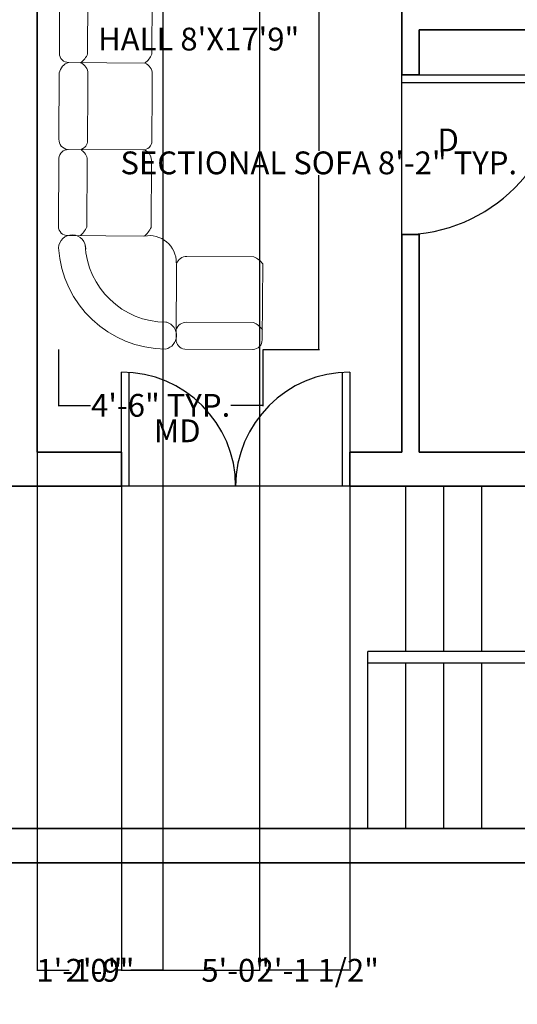
# Model space of a CAD drawing. Units: inches. Extents: x -26 to 575, y -18 to 513.
# Tile 15 of 28: x 274 to 405, y -18 to 241. Entities that reach past the tile are written whole.
import ezdxf

# ---------------------------------------------------------------- set-up
doc = ezdxf.new("R2010")
doc.units = ezdxf.units.IN
doc.header["$MEASUREMENT"] = 0
for name, color, linetype, lineweight in [('A-ANNO-DIMS', 2, 'Continuous', 18), ('A-ANNO-TEXT', 7, 'Continuous', 18), ('A-AREA-IDEN', 7, 'Continuous', 18), ('A-DOOR', 3, 'Continuous', 25), ('A-FLOR-STRS', 7, 'Continuous', 25), ('A-WALL', 7, 'Continuous', 35), ('Furniture', 8, 'Continuous', 15)]:
    doc.layers.add(name, color=color, linetype=linetype, lineweight=lineweight)
doc.styles.get("Standard").update_dxf_attribs({"font": 'arial.ttf', "height": 6})
doc.dimstyles.get("Standard").update_dxf_attribs({"dimtxt": 6, "dimasz": 0.18, "dimexe": 0.18, "dimexo": 0.0625, "dimgap": 0.09, "dimtad": 0, "dimtih": 1, "dimtoh": 1, "dimzin": 0, "dimdsep": 46, "dimlunit": 3, "dimtxsty": 'Standard', "dimcen": 0.09, "dimadec": 0, "dimazin": 0, "dimtfac": 1, "dimtofl": 0, "dimtmove": 0, "dimatfit": 3, "dimfxl": 1, "dimtolj": 1, "dimtzin": 0, "dimarcsym": 0})

# ---------------------------------------------------------------- blocks, each defined once
blk = doc.blocks.new('SOFA-L-SECTIONAL')
for p, q in [((0.33, 95.83, -13.5), (0.23, 77.86, -13.5)), ((22.74, 97.99, -13.5), (2.82, 98.09, -13.5)), ((7.68, 77.72, -13.5), (7.77, 95.38, -13.5)), ((24.59, 77.63, -13.5), (24.69, 95.29, -13.5)), ((2.7, 75.47, -13.5), (22.72, 75.27, -13.5)), ((0.21, 72.7, -13.5), (0.12, 55.25, -13.5)), ((7.74, 68.12, -13.5), (7.76, 72.56, -13.5)), ((24.65, 68.03, -13.5), (24.67, 72.47, -13.5)), ((7.67, 54.9, -13.5), (7.74, 68.12, -13.5)), ((24.58, 54.81, -13.5), (24.65, 68.03, -13.5)), ((2.38, 52.55, -13.5), (22.19, 52.45, -13.5)), ((22.5, 52.45, -13.5), (2.58, 52.55, -13.5)), ((0.09, 50.29, -13.5), (0, 32.32, -13.5)), ((7.45, 32.18, -13.5), (7.54, 49.84, -13.5)), ((24.36, 32.09, -13.5), (24.45, 49.75, -13.5)), ((2.47, 29.93, -13.5), (22.49, 29.73, -13.5)), ((51.42, 24.36, -13.5), (33.76, 24.45, -13.5)), ((31.06, 22.5, -13.5), (30.96, 2.58, -13.5)), ((53.78, 22.49, -13.5), (53.58, 2.47, -13.5)), ((28.5, 7.13, -13.5), (28.26, 7.13, -13.5)), ((30.97, 5.19, -13.5), (30.97, 5.12, -13.5)), ((51.33, 7.05, -13.5), (33.67, 7.14, -13.5)), ((33.22, 0.09, -13.5), (51.19, 0, -13.5))]:
    blk.add_line(p, q)
for centre, radius, start, end in [((2.8, 95.6, -13.5), 2.49, 89.7045, 174.7543), ((4.96, 95.39, -13.5), 2.82, 359.7045, 63.7788), ((21.87, 95.31, -13.5), 2.82, 359.7045, 71.9933), ((2.61, 77.85, -13.5), 2.38, 179.7045, 272.1133), ((2.36, 80.01, -13.5), 5.79, 306.5883, 336.7547), ((3.67, 72.1, -13.5), 3.51, 105.9725, 170.1982), ((4.8, 72.57, -13.5), 2.96, 359.7045, 69.9456), ((19.27, 79.92, -13.5), 5.79, 306.5883, 336.7547), ((21.71, 72.48, -13.5), 2.96, 359.7045, 69.9456), ((2.84, 55.23, -13.5), 2.72, 179.7045, 260.1487), ((5.3, 54.91, -13.5), 2.37, 286.4623, 359.7335), ((22.21, 54.82, -13.5), 2.37, 269.7045, 359.7335), ((2.57, 50.06, -13.5), 2.49, 89.7045, 174.7543), ((4.72, 49.86, -13.5), 2.82, 359.7045, 63.7788), ((21.63, 49.77, -13.5), 2.82, 359.7045, 71.9933), ((2.38, 32.31, -13.5), 2.38, 179.7045, 272.1133), ((2.12, 34.47, -13.5), 5.79, 306.5883, 336.7547), ((19.04, 34.38, -13.5), 5.79, 306.5883, 336.7547), ((3.6, 26.52, -13.5), 3.6, 357.7166, 177.7166), ((23.89, 22.8, -13.5), 7.12, 359.7045, 100.3051), ((28.37, 28.51, -13.5), 28.42, 183.6915, 269.6528), ((28.37, 28.51, -13.5), 21.38, 182.6205, 269.7045), ((33.74, 21.63, -13.5), 2.82, 89.7045, 161.9933), ((49.13, 19.04, -13.5), 5.79, 36.5883, 66.7547), ((27.43, 3.65, -13.5), 3.64, 282.1306, 72.938), ((33.65, 4.32, -13.5), 2.82, 89.7045, 161.9933), ((49.04, 1.73, -13.5), 5.79, 36.5883, 66.7547), ((33.45, 2.57, -13.5), 2.49, 179.7045, 264.7543), ((51.2, 2.38, -13.5), 2.38, 269.7045, 2.1133)]:
    blk.add_arc(centre, radius, start, end)
blk = doc.blocks.new('DOOR-SWING-42IN')
for p, q in [((0, 0), (0, 42)), ((2, 0), (2, 42)), ((42, 0), (0, 0))]:
    blk.add_line(p, q)
blk.add_arc((0, 0), 42, 0, 90)
blk = doc.blocks.new('*D26')
at = {"layer": 'A-ANNO-DIMS', "color": 0, "lineweight": -2, "transparency": 16777216}
for p, q in [((337.63, 252.61), (352.46, 252.61)), ((352.28, 252.43), (352.28, 206.75)), ((352.28, 154.69), (352.28, 200.36)), ((337.63, 154.51), (352.46, 154.51))]:
    blk.add_line(p, q, dxfattribs=at)
at = {"layer": 'A-ANNO-DIMS', "color": 0, "transparency": 16777216}
for points in [[(352.25, 252.43), (352.31, 252.43), (352.28, 252.61)], [(352.25, 154.69), (352.31, 154.69), (352.28, 154.51)]]:
    blk.add_solid(points, dxfattribs=at)
at = {"layer": 'Defpoints', "color": 0, "transparency": 16777216}
for p in [(337.57, 252.61), (352.28, 252.61), (337.57, 154.51)]:
    blk.add_point(p, dxfattribs=at)
at = {"layer": 'A-ANNO-DIMS', "color": 0, "transparency": 16777216, "insert": (352.28, 203.56), "char_height": 6, "attachment_point": 5}
blk.add_mtext('\\A1;SECTIONAL SOFA 8\'-2" TYP.', dxfattribs=at)
blk = doc.blocks.new('*D27')
at = {"layer": 'A-ANNO-DIMS', "color": 0, "lineweight": -2, "transparency": 16777216}
for p, q in [((283.78, 154.45), (283.78, 139.61)), ((337.57, 154.45), (337.57, 139.61)), ((283.96, 139.79), (292.18, 139.79)), ((337.39, 139.79), (329.17, 139.79))]:
    blk.add_line(p, q, dxfattribs=at)
at = {"layer": 'A-ANNO-DIMS', "color": 0, "transparency": 16777216}
for points in [[(283.96, 139.82), (283.96, 139.76), (283.78, 139.79)], [(337.39, 139.82), (337.39, 139.76), (337.57, 139.79)]]:
    blk.add_solid(points, dxfattribs=at)
at = {"layer": 'Defpoints', "color": 0, "transparency": 16777216}
for p in [(283.78, 154.51), (337.57, 154.51), (337.57, 139.79)]:
    blk.add_point(p, dxfattribs=at)
at = {"layer": 'A-ANNO-DIMS', "color": 0, "transparency": 16777216, "insert": (310.67, 139.79), "char_height": 6, "attachment_point": 5}
blk.add_mtext('\\A1;4\'-6" TYP.', dxfattribs=at)
blk = doc.blocks.new('*D31')
at = {"layer": 'A-ANNO-DIMS', "color": 0, "lineweight": -2, "transparency": 16777216}
for p, q in [((311.29, 466.45), (311.29, -8.97)), ((336.72, 466.45), (336.72, -8.97)), ((311.47, -8.79), (336.54, -8.79)), ((336.72, -8.79), (336.9, -8.79))]:
    blk.add_line(p, q, dxfattribs=at)
at = {"layer": 'A-ANNO-DIMS', "color": 0, "transparency": 16777216}
for points in [[(311.47, -8.76), (311.47, -8.82), (311.29, -8.79)], [(336.54, -8.76), (336.54, -8.82), (336.72, -8.79)]]:
    blk.add_solid(points, dxfattribs=at)
at = {"layer": 'Defpoints', "color": 0, "transparency": 16777216}
for p in [(311.29, 466.51), (336.72, 466.51), (336.72, -8.79)]:
    blk.add_point(p, dxfattribs=at)
at = {"layer": 'A-ANNO-DIMS', "color": 0, "transparency": 16777216, "insert": (352.01, -8.79), "char_height": 6, "attachment_point": 5}
blk.add_mtext('\\A1;2\'-1 1/2"', dxfattribs=at)
blk = doc.blocks.new('*D34')
at = {"layer": 'A-ANNO-DIMS', "color": 0, "lineweight": -2, "transparency": 16777216}
for p, q in [((300.41, 118.45), (300.41, -8.97)), ((360.41, 118.45), (360.41, -8.97)), ((300.59, -8.79), (322.34, -8.79)), ((360.23, -8.79), (338.47, -8.79))]:
    blk.add_line(p, q, dxfattribs=at)
at = {"layer": 'A-ANNO-DIMS', "color": 0, "transparency": 16777216}
for points in [[(300.59, -8.76), (300.59, -8.82), (300.41, -8.79)], [(360.23, -8.76), (360.23, -8.82), (360.41, -8.79)]]:
    blk.add_solid(points, dxfattribs=at)
at = {"layer": 'Defpoints', "color": 0, "transparency": 16777216}
for p in [(300.41, 118.51), (360.41, 118.51), (360.41, -8.79)]:
    blk.add_point(p, dxfattribs=at)
at = {"layer": 'A-ANNO-DIMS', "color": 0, "transparency": 16777216, "insert": (330.41, -8.79), "char_height": 6, "attachment_point": 5}
blk.add_mtext('\\A1;5\'-0"', dxfattribs=at)
blk = doc.blocks.new('*D41')
at = {"layer": 'A-ANNO-DIMS', "color": 0, "lineweight": -2, "transparency": 16777216}
for p, q in [((278.18, 127.45), (278.18, -8.97)), ((300.41, 118.45), (300.41, -8.97)), ((278.36, -8.79), (279.18, -8.79)), ((300.23, -8.79), (299.41, -8.79))]:
    blk.add_line(p, q, dxfattribs=at)
at = {"layer": 'A-ANNO-DIMS', "color": 0, "transparency": 16777216}
for points in [[(278.36, -8.76), (278.36, -8.82), (278.18, -8.79)], [(300.23, -8.76), (300.23, -8.82), (300.41, -8.79)]]:
    blk.add_solid(points, dxfattribs=at)
at = {"layer": 'Defpoints', "color": 0, "transparency": 16777216}
for p in [(278.18, 127.51), (300.41, 118.51), (300.41, -8.79)]:
    blk.add_point(p, dxfattribs=at)
at = {"layer": 'A-ANNO-DIMS', "color": 0, "transparency": 16777216, "insert": (289.29, -8.79), "char_height": 6, "attachment_point": 5}
blk.add_mtext('\\A1;1\'-10"', dxfattribs=at)
blk = doc.blocks.new('*D47')
at = {"layer": 'A-ANNO-DIMS', "color": 0, "lineweight": -2, "transparency": 16777216}
for p, q in [((278.18, 466.45), (278.18, -8.97)), ((311.29, 466.45), (311.29, -8.97)), ((278.36, -8.79), (286.62, -8.79)), ((311.11, -8.79), (302.85, -8.79))]:
    blk.add_line(p, q, dxfattribs=at)
at = {"layer": 'A-ANNO-DIMS', "color": 0, "transparency": 16777216}
for points in [[(278.36, -8.76), (278.36, -8.82), (278.18, -8.79)], [(311.11, -8.76), (311.11, -8.82), (311.29, -8.79)]]:
    blk.add_solid(points, dxfattribs=at)
at = {"layer": 'Defpoints', "color": 0, "transparency": 16777216}
for p in [(278.18, 466.51), (311.29, 466.51), (311.29, -8.79)]:
    blk.add_point(p, dxfattribs=at)
at = {"layer": 'A-ANNO-DIMS', "color": 0, "transparency": 16777216, "insert": (294.73, -8.79), "char_height": 6, "attachment_point": 5}
blk.add_mtext('\\A1;2\'-9"', dxfattribs=at)

msp = doc.modelspace()

# ---------------------------------------------------------------- linework, layer by layer
at = {"layer": 'A-DOOR'}
for p, q in [((300.409, 118.508), (300.409, 148.508)), ((302.409, 118.508), (302.409, 148.508)), ((358.409, 148.508), (358.409, 118.508)), ((360.409, 148.508), (360.409, 118.508)), ((360.409, 118.508), (300.409, 118.508))]:
    msp.add_line(p, q, dxfattribs=at)
for centre, start, end in [((300.409, 118.508), 0, 90), ((360.409, 118.508), 90, 180)]:
    msp.add_arc(centre, 30, start, end, dxfattribs=at)
at = {"layer": 'A-FLOR-STRS'}
for p, q in [((375.177, 75.008), (375.177, 118.508)), ((385.177, 75.008), (385.177, 118.508)), ((395.177, 75.008), (395.177, 118.508)), ((465.177, 75.008), (365.177, 75.008)), ((365.177, 28.508), (365.177, 75.008)), ((465.177, 72.008), (365.177, 72.008)), ((375.177, 28.508), (375.177, 72.008)), ((385.177, 28.508), (385.177, 72.008)), ((395.177, 28.508), (395.177, 72.008))]:
    msp.add_line(p, q, dxfattribs=at)
at = {"layer": 'A-WALL'}
for p, q in [((278.177, 127.508), (278.177, 330.008)), ((374.177, 226.702), (374.177, 298.508)), ((513.177, 238.508), (378.677, 238.508)), ((378.677, 226.702), (378.677, 238.508)), ((378.677, 226.702), (374.177, 226.702)), ((374.177, 127.508), (374.177, 184.702)), ((378.677, 184.702), (374.177, 184.702)), ((378.677, 127.508), (378.677, 184.702)), ((300.409, 127.508), (278.177, 127.508)), ((300.409, 118.508), (300.409, 127.508)), ((374.177, 127.508), (360.409, 127.508)), ((360.409, 118.508), (360.409, 127.508)), ((513.177, 127.508), (378.677, 127.508)), ((300.409, 118.508), (27.177, 118.508)), ((522.177, 118.508), (360.409, 118.508)), ((27.177, 28.508), (513.177, 28.508))]:
    msp.add_line(p, q, dxfattribs=at)
msp.add_lwpolyline([(18.177, 19.508), (522.177, 19.508), (522.177, 475.508), (18.177, 475.508)], close=True, dxfattribs=at)

# ---------------------------------------------------------------- block references
at = {"layer": 'A-DOOR', "rotation": 270}
msp.add_blockref('DOOR-SWING-42IN', (374.177, 226.702), dxfattribs=at)
at = {"layer": 'Furniture'}
msp.add_blockref('SOFA-L-SECTIONAL', (283.784, 154.512), dxfattribs=at)

# ---------------------------------------------------------------- texts
at = {"layer": 'A-ANNO-TEXT'}
for s, p in [('D', (383.516, 206.6)), ('MD', (308.904, 130.096))]:
    msp.add_text(s, height=6, rotation=0.00167, dxfattribs=at).set_placement(p)
at = {"layer": 'A-AREA-IDEN'}
msp.add_text('HALL 8\'X17\'9"', height=6, rotation=0.00167, dxfattribs=at).set_placement((294.201, 233.117))

# ---------------------------------------------------------------- dimensions: what is measured, and where the dimension line sits
at = {"layer": 'A-ANNO-DIMS'}
for base, p1, p2, picture, middle in [((311.292, -8.792), (278.177, 466.508), (311.292, 466.508), '*D47', (294.735, -8.792)), ((336.72, -8.792), (311.292, 466.508), (336.72, 466.508), '*D31', (352.006, -8.792)), ((300.409, -8.792), (278.177, 127.508), (300.409, 118.508), '*D41', (289.293, -8.792)), ((360.409, -8.792), (300.409, 118.508), (360.409, 118.508), '*D34', (330.409, -8.792))]:
    dim = msp.add_linear_dim(base=base, p1=p1, p2=p2, dimstyle='Standard', override={"dimdec": 1, "dimlfac": 1, "dimrnd": 0, "dimzin": 1, "dimdsep": 46, "dimlunit": 4, "dimfrac": 2}, dxfattribs=at)
    dim.commit()
    dim.dimension.update_dxf_attribs({"geometry": picture, "text_midpoint": middle})
dim = msp.add_linear_dim(base=(352.281, 252.609), p1=(337.566, 154.509), p2=(337.566, 252.609), angle=90, text='SECTIONAL SOFA <> TYP.', dimstyle='Standard', override={"dimdec": 1, "dimlfac": 1, "dimrnd": 0, "dimzin": 1, "dimdsep": 46, "dimlunit": 4, "dimfrac": 2}, dxfattribs=at)
dim.commit()
dim.dimension.update_dxf_attribs({"geometry": '*D26', "text_midpoint": (352.281, 203.559)})
dim = msp.add_linear_dim(base=(337.566, 139.794), p1=(283.781, 154.509), p2=(337.566, 154.509), text='<> TYP.', dimstyle='Standard', override={"dimdec": 1, "dimlfac": 1, "dimrnd": 0, "dimzin": 1, "dimdsep": 46, "dimlunit": 4, "dimfrac": 2}, dxfattribs=at)
dim.commit()
dim.dimension.update_dxf_attribs({"geometry": '*D27', "text_midpoint": (310.673, 139.794)})

doc.saveas('drawing.dxf')
